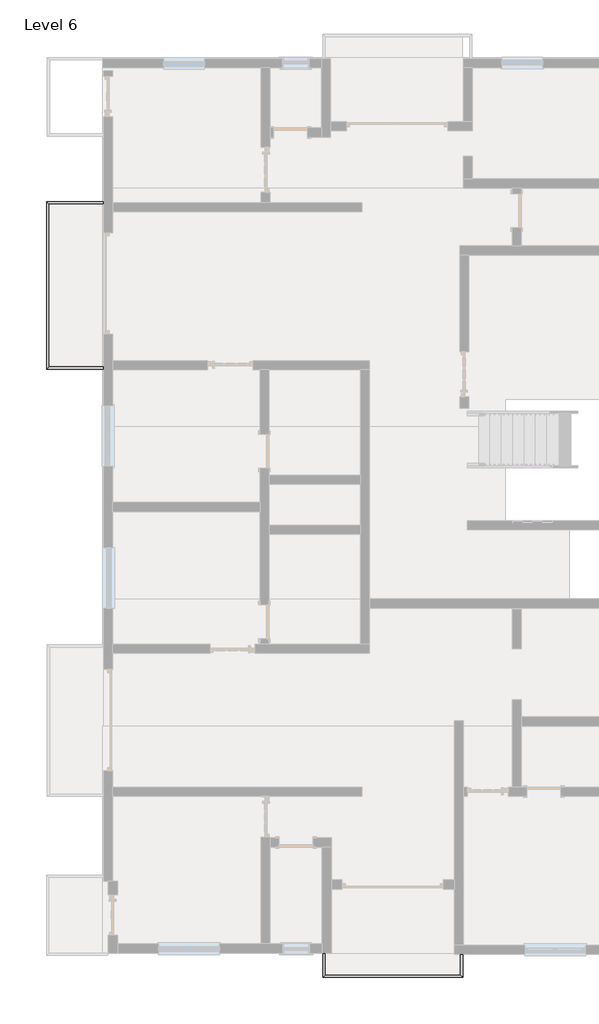
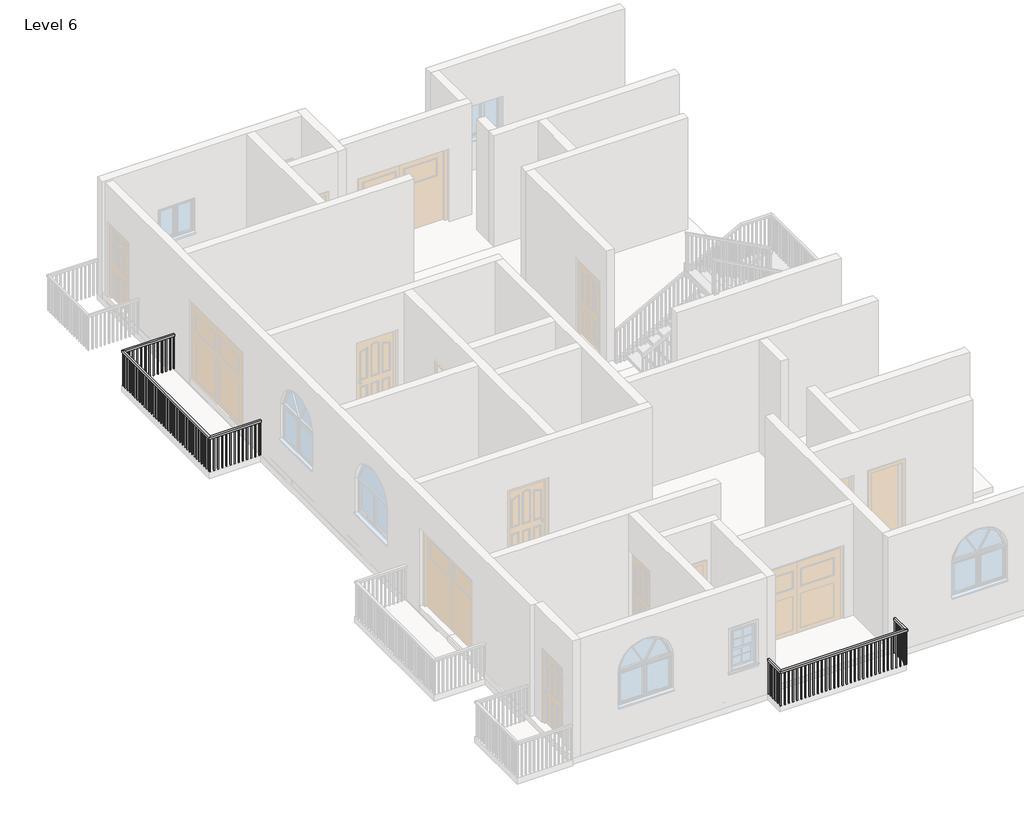
# One storey, part 4 of 7: 2 railings.
"""IFC4 building model written with IfcOpenShell, lengths in millimetres."""

from ifc_helpers import new_model, si_unit, frame, origin, place, context, project, spatial, polyline, outline, extrude, faceted_brep, element, save

model = new_model("IFC4")

# Units and contexts
model_context = context("Model", 3, world=origin())
ifc_project = project(units=[si_unit("LENGTHUNIT", "METRE", prefix="MILLI")], contexts=[model_context])

# Site, building, storey
site = spatial("IfcSite", under=ifc_project)
building = spatial("IfcBuilding", under=site)
storey = spatial("IfcBuildingStorey", under=building, Name="Level 6", Elevation=15240.0)

# Railings
placement = place(None, origin())
element("IfcRailing", 1, ObjectType="Handrail - Rectangular", at=placement, inside=storey, context=model_context, shape_type="SolidModel", body=[
    faceted_brep([(-1375.8109037, -10612.9037749, 16154.4), (-1375.8109037, -10612.9037749, 16103.6), (-1426.6109037, -10612.9037749, 16103.6), (-1426.6109037, -10612.9037749, 16154.4), (-1375.8109037, -11108.2037749, 16154.4), (-1375.8109037, -11108.2037749, 16103.6), (-1426.6109037, -11159.0037749, 16103.6), (-1426.6109037, -11159.0037749, 16154.4), (1659.4890963, -11108.2037749, 16154.4), (1659.4890963, -11108.2037749, 16103.6), (1710.2890963, -11159.0037749, 16103.6), (1710.2890963, -11159.0037749, 16154.4), (1659.4890963, -10638.3037749, 16154.4), (1710.2890963, -10638.3037749, 16154.4), (1710.2890963, -10638.3037749, 16103.6), (1659.4890963, -10638.3037749, 16103.6)], [[[0, 1, 2, 3]], [[1, 0, 4, 5]], [[2, 1, 5, 6]], [[3, 2, 6, 7]], [[0, 3, 7, 4]], [[5, 4, 8, 9]], [[6, 5, 9, 10]], [[7, 6, 10, 11]], [[4, 7, 11, 8]], [[12, 13, 14, 15]], [[9, 8, 12, 15]], [[10, 9, 15, 14]], [[11, 10, 14, 13]], [[8, 11, 13, 12]]]),
    extrude(outline(polyline([(1694.4140963, -10736.7287749), (1675.3640963, -10736.7287749), (1675.3640963, -10717.6787749), (1694.4140963, -10717.6787749), (1694.4140963, -10736.7287749)])), frame((0.0, 0.0, 15240.0), z_axis=(0.0, 0.0, 1.0), x_axis=(1.0, 0.0, 0.0)), (0.0, 0.0, 1.0), 863.6),
    extrude(outline(polyline([(1694.4140963, -10838.3287749), (1675.3640963, -10838.3287749), (1675.3640963, -10819.2787749), (1694.4140963, -10819.2787749), (1694.4140963, -10838.3287749)])), frame((0.0, 0.0, 15240.0), z_axis=(0.0, 0.0, 1.0), x_axis=(1.0, 0.0, 0.0)), (0.0, 0.0, 1.0), 863.6),
    extrude(outline(polyline([(1694.4140963, -10939.9287749), (1675.3640963, -10939.9287749), (1675.3640963, -10920.8787749), (1694.4140963, -10920.8787749), (1694.4140963, -10939.9287749)])), frame((0.0, 0.0, 15240.0), z_axis=(0.0, 0.0, 1.0), x_axis=(1.0, 0.0, 0.0)), (0.0, 0.0, 1.0), 863.6),
    extrude(outline(polyline([(1694.4140963, -11041.5287749), (1675.3640963, -11041.5287749), (1675.3640963, -11022.4787749), (1694.4140963, -11022.4787749), (1694.4140963, -11041.5287749)])), frame((0.0, 0.0, 15240.0), z_axis=(0.0, 0.0, 1.0), x_axis=(1.0, 0.0, 0.0)), (0.0, 0.0, 1.0), 863.6),
    extrude(outline(polyline([(1637.2640963, -11143.1287749), (1637.2640963, -11124.0787749), (1656.3140963, -11124.0787749), (1656.3140963, -11143.1287749), (1637.2640963, -11143.1287749)])), frame((0.0, 0.0, 15240.0), z_axis=(0.0, 0.0, 1.0), x_axis=(1.0, 0.0, 0.0)), (0.0, 0.0, 1.0), 863.6),
    extrude(outline(polyline([(1535.6640963, -11143.1287749), (1535.6640963, -11124.0787749), (1554.7140963, -11124.0787749), (1554.7140963, -11143.1287749), (1535.6640963, -11143.1287749)])), frame((0.0, 0.0, 15240.0), z_axis=(0.0, 0.0, 1.0), x_axis=(1.0, 0.0, 0.0)), (0.0, 0.0, 1.0), 863.6),
    extrude(outline(polyline([(1434.0640963, -11143.1287749), (1434.0640963, -11124.0787749), (1453.1140963, -11124.0787749), (1453.1140963, -11143.1287749), (1434.0640963, -11143.1287749)])), frame((0.0, 0.0, 15240.0), z_axis=(0.0, 0.0, 1.0), x_axis=(1.0, 0.0, 0.0)), (0.0, 0.0, 1.0), 863.6),
    extrude(outline(polyline([(1332.4640963, -11143.1287749), (1332.4640963, -11124.0787749), (1351.5140963, -11124.0787749), (1351.5140963, -11143.1287749), (1332.4640963, -11143.1287749)])), frame((0.0, 0.0, 15240.0), z_axis=(0.0, 0.0, 1.0), x_axis=(1.0, 0.0, 0.0)), (0.0, 0.0, 1.0), 863.6),
    extrude(outline(polyline([(1230.8640963, -11143.1287749), (1230.8640963, -11124.0787749), (1249.9140963, -11124.0787749), (1249.9140963, -11143.1287749), (1230.8640963, -11143.1287749)])), frame((0.0, 0.0, 15240.0), z_axis=(0.0, 0.0, 1.0), x_axis=(1.0, 0.0, 0.0)), (0.0, 0.0, 1.0), 863.6),
    extrude(outline(polyline([(1129.2640963, -11143.1287749), (1129.2640963, -11124.0787749), (1148.3140963, -11124.0787749), (1148.3140963, -11143.1287749), (1129.2640963, -11143.1287749)])), frame((0.0, 0.0, 15240.0), z_axis=(0.0, 0.0, 1.0), x_axis=(1.0, 0.0, 0.0)), (0.0, 0.0, 1.0), 863.6),
    extrude(outline(polyline([(1027.6640963, -11143.1287749), (1027.6640963, -11124.0787749), (1046.7140963, -11124.0787749), (1046.7140963, -11143.1287749), (1027.6640963, -11143.1287749)])), frame((0.0, 0.0, 15240.0), z_axis=(0.0, 0.0, 1.0), x_axis=(1.0, 0.0, 0.0)), (0.0, 0.0, 1.0), 863.6),
    extrude(outline(polyline([(926.0640963, -11143.1287749), (926.0640963, -11124.0787749), (945.1140963, -11124.0787749), (945.1140963, -11143.1287749), (926.0640963, -11143.1287749)])), frame((0.0, 0.0, 15240.0), z_axis=(0.0, 0.0, 1.0), x_axis=(1.0, 0.0, 0.0)), (0.0, 0.0, 1.0), 863.6),
    extrude(outline(polyline([(824.4640963, -11143.1287749), (824.4640963, -11124.0787749), (843.5140963, -11124.0787749), (843.5140963, -11143.1287749), (824.4640963, -11143.1287749)])), frame((0.0, 0.0, 15240.0), z_axis=(0.0, 0.0, 1.0), x_axis=(1.0, 0.0, 0.0)), (0.0, 0.0, 1.0), 863.6),
    extrude(outline(polyline([(722.8640963, -11143.1287749), (722.8640963, -11124.0787749), (741.9140963, -11124.0787749), (741.9140963, -11143.1287749), (722.8640963, -11143.1287749)])), frame((0.0, 0.0, 15240.0), z_axis=(0.0, 0.0, 1.0), x_axis=(1.0, 0.0, 0.0)), (0.0, 0.0, 1.0), 863.6),
    extrude(outline(polyline([(621.2640963, -11143.1287749), (621.2640963, -11124.0787749), (640.3140963, -11124.0787749), (640.3140963, -11143.1287749), (621.2640963, -11143.1287749)])), frame((0.0, 0.0, 15240.0), z_axis=(0.0, 0.0, 1.0), x_axis=(1.0, 0.0, 0.0)), (0.0, 0.0, 1.0), 863.6),
    extrude(outline(polyline([(519.6640963, -11143.1287749), (519.6640963, -11124.0787749), (538.7140963, -11124.0787749), (538.7140963, -11143.1287749), (519.6640963, -11143.1287749)])), frame((0.0, 0.0, 15240.0), z_axis=(0.0, 0.0, 1.0), x_axis=(1.0, 0.0, 0.0)), (0.0, 0.0, 1.0), 863.6),
    extrude(outline(polyline([(418.0640963, -11143.1287749), (418.0640963, -11124.0787749), (437.1140963, -11124.0787749), (437.1140963, -11143.1287749), (418.0640963, -11143.1287749)])), frame((0.0, 0.0, 15240.0), z_axis=(0.0, 0.0, 1.0), x_axis=(1.0, 0.0, 0.0)), (0.0, 0.0, 1.0), 863.6),
    extrude(outline(polyline([(316.4640963, -11143.1287749), (316.4640963, -11124.0787749), (335.5140963, -11124.0787749), (335.5140963, -11143.1287749), (316.4640963, -11143.1287749)])), frame((0.0, 0.0, 15240.0), z_axis=(0.0, 0.0, 1.0), x_axis=(1.0, 0.0, 0.0)), (0.0, 0.0, 1.0), 863.6),
    extrude(outline(polyline([(214.8640963, -11143.1287749), (214.8640963, -11124.0787749), (233.9140963, -11124.0787749), (233.9140963, -11143.1287749), (214.8640963, -11143.1287749)])), frame((0.0, 0.0, 15240.0), z_axis=(0.0, 0.0, 1.0), x_axis=(1.0, 0.0, 0.0)), (0.0, 0.0, 1.0), 863.6),
    extrude(outline(polyline([(113.2640963, -11143.1287749), (113.2640963, -11124.0787749), (132.3140963, -11124.0787749), (132.3140963, -11143.1287749), (113.2640963, -11143.1287749)])), frame((0.0, 0.0, 15240.0), z_axis=(0.0, 0.0, 1.0), x_axis=(1.0, 0.0, 0.0)), (0.0, 0.0, 1.0), 863.6),
    extrude(outline(polyline([(11.6640963, -11143.1287749), (11.6640963, -11124.0787749), (30.7140963, -11124.0787749), (30.7140963, -11143.1287749), (11.6640963, -11143.1287749)])), frame((0.0, 0.0, 15240.0), z_axis=(0.0, 0.0, 1.0), x_axis=(1.0, 0.0, 0.0)), (0.0, 0.0, 1.0), 863.6),
    extrude(outline(polyline([(-89.9359037, -11143.1287749), (-89.9359037, -11124.0787749), (-70.8859037, -11124.0787749), (-70.8859037, -11143.1287749), (-89.9359037, -11143.1287749)])), frame((0.0, 0.0, 15240.0), z_axis=(0.0, 0.0, 1.0), x_axis=(1.0, 0.0, 0.0)), (0.0, 0.0, 1.0), 863.6),
    extrude(outline(polyline([(-191.5359037, -11143.1287749), (-191.5359037, -11124.0787749), (-172.4859037, -11124.0787749), (-172.4859037, -11143.1287749), (-191.5359037, -11143.1287749)])), frame((0.0, 0.0, 15240.0), z_axis=(0.0, 0.0, 1.0), x_axis=(1.0, 0.0, 0.0)), (0.0, 0.0, 1.0), 863.6),
    extrude(outline(polyline([(-293.1359037, -11143.1287749), (-293.1359037, -11124.0787749), (-274.0859037, -11124.0787749), (-274.0859037, -11143.1287749), (-293.1359037, -11143.1287749)])), frame((0.0, 0.0, 15240.0), z_axis=(0.0, 0.0, 1.0), x_axis=(1.0, 0.0, 0.0)), (0.0, 0.0, 1.0), 863.6),
    extrude(outline(polyline([(-394.7359037, -11143.1287749), (-394.7359037, -11124.0787749), (-375.6859037, -11124.0787749), (-375.6859037, -11143.1287749), (-394.7359037, -11143.1287749)])), frame((0.0, 0.0, 15240.0), z_axis=(0.0, 0.0, 1.0), x_axis=(1.0, 0.0, 0.0)), (0.0, 0.0, 1.0), 863.6),
    extrude(outline(polyline([(-496.3359037, -11143.1287749), (-496.3359037, -11124.0787749), (-477.2859037, -11124.0787749), (-477.2859037, -11143.1287749), (-496.3359037, -11143.1287749)])), frame((0.0, 0.0, 15240.0), z_axis=(0.0, 0.0, 1.0), x_axis=(1.0, 0.0, 0.0)), (0.0, 0.0, 1.0), 863.6),
    extrude(outline(polyline([(-597.9359037, -11143.1287749), (-597.9359037, -11124.0787749), (-578.8859037, -11124.0787749), (-578.8859037, -11143.1287749), (-597.9359037, -11143.1287749)])), frame((0.0, 0.0, 15240.0), z_axis=(0.0, 0.0, 1.0), x_axis=(1.0, 0.0, 0.0)), (0.0, 0.0, 1.0), 863.6),
    extrude(outline(polyline([(-699.5359037, -11143.1287749), (-699.5359037, -11124.0787749), (-680.4859037, -11124.0787749), (-680.4859037, -11143.1287749), (-699.5359037, -11143.1287749)])), frame((0.0, 0.0, 15240.0), z_axis=(0.0, 0.0, 1.0), x_axis=(1.0, 0.0, 0.0)), (0.0, 0.0, 1.0), 863.6),
    extrude(outline(polyline([(-801.1359037, -11143.1287749), (-801.1359037, -11124.0787749), (-782.0859037, -11124.0787749), (-782.0859037, -11143.1287749), (-801.1359037, -11143.1287749)])), frame((0.0, 0.0, 15240.0), z_axis=(0.0, 0.0, 1.0), x_axis=(1.0, 0.0, 0.0)), (0.0, 0.0, 1.0), 863.6),
    extrude(outline(polyline([(-902.7359037, -11143.1287749), (-902.7359037, -11124.0787749), (-883.6859037, -11124.0787749), (-883.6859037, -11143.1287749), (-902.7359037, -11143.1287749)])), frame((0.0, 0.0, 15240.0), z_axis=(0.0, 0.0, 1.0), x_axis=(1.0, 0.0, 0.0)), (0.0, 0.0, 1.0), 863.6),
    extrude(outline(polyline([(-1004.3359037, -11143.1287749), (-1004.3359037, -11124.0787749), (-985.2859037, -11124.0787749), (-985.2859037, -11143.1287749), (-1004.3359037, -11143.1287749)])), frame((0.0, 0.0, 15240.0), z_axis=(0.0, 0.0, 1.0), x_axis=(1.0, 0.0, 0.0)), (0.0, 0.0, 1.0), 863.6),
    extrude(outline(polyline([(-1105.9359037, -11143.1287749), (-1105.9359037, -11124.0787749), (-1086.8859037, -11124.0787749), (-1086.8859037, -11143.1287749), (-1105.9359037, -11143.1287749)])), frame((0.0, 0.0, 15240.0), z_axis=(0.0, 0.0, 1.0), x_axis=(1.0, 0.0, 0.0)), (0.0, 0.0, 1.0), 863.6),
    extrude(outline(polyline([(-1207.5359037, -11143.1287749), (-1207.5359037, -11124.0787749), (-1188.4859037, -11124.0787749), (-1188.4859037, -11143.1287749), (-1207.5359037, -11143.1287749)])), frame((0.0, 0.0, 15240.0), z_axis=(0.0, 0.0, 1.0), x_axis=(1.0, 0.0, 0.0)), (0.0, 0.0, 1.0), 863.6),
    extrude(outline(polyline([(-1309.1359037, -11143.1287749), (-1309.1359037, -11124.0787749), (-1290.0859037, -11124.0787749), (-1290.0859037, -11143.1287749), (-1309.1359037, -11143.1287749)])), frame((0.0, 0.0, 15240.0), z_axis=(0.0, 0.0, 1.0), x_axis=(1.0, 0.0, 0.0)), (0.0, 0.0, 1.0), 863.6),
    extrude(outline(polyline([(-1410.7359037, -11111.3787749), (-1391.6859037, -11111.3787749), (-1391.6859037, -11130.4287749), (-1410.7359037, -11130.4287749), (-1410.7359037, -11111.3787749)])), frame((0.0, 0.0, 15240.0), z_axis=(0.0, 0.0, 1.0), x_axis=(1.0, 0.0, 0.0)), (0.0, 0.0, 1.0), 863.6),
    extrude(outline(polyline([(-1410.7359037, -11009.7787749), (-1391.6859037, -11009.7787749), (-1391.6859037, -11028.8287749), (-1410.7359037, -11028.8287749), (-1410.7359037, -11009.7787749)])), frame((0.0, 0.0, 15240.0), z_axis=(0.0, 0.0, 1.0), x_axis=(1.0, 0.0, 0.0)), (0.0, 0.0, 1.0), 863.6),
    extrude(outline(polyline([(-1410.7359037, -10908.1787749), (-1391.6859037, -10908.1787749), (-1391.6859037, -10927.2287749), (-1410.7359037, -10927.2287749), (-1410.7359037, -10908.1787749)])), frame((0.0, 0.0, 15240.0), z_axis=(0.0, 0.0, 1.0), x_axis=(1.0, 0.0, 0.0)), (0.0, 0.0, 1.0), 863.6),
    extrude(outline(polyline([(-1410.7359037, -10806.5787749), (-1391.6859037, -10806.5787749), (-1391.6859037, -10825.6287749), (-1410.7359037, -10825.6287749), (-1410.7359037, -10806.5787749)])), frame((0.0, 0.0, 15240.0), z_axis=(0.0, 0.0, 1.0), x_axis=(1.0, 0.0, 0.0)), (0.0, 0.0, 1.0), 863.6),
    extrude(outline(polyline([(-1410.7359037, -10704.9787749), (-1391.6859037, -10704.9787749), (-1391.6859037, -10724.0287749), (-1410.7359037, -10724.0287749), (-1410.7359037, -10704.9787749)])), frame((0.0, 0.0, 15240.0), z_axis=(0.0, 0.0, 1.0), x_axis=(1.0, 0.0, 0.0)), (0.0, 0.0, 1.0), 863.6),
    extrude(outline(polyline([(1675.3640963, -11143.1287749), (1675.3640963, -11124.0787749), (1694.4140963, -11124.0787749), (1694.4140963, -11143.1287749), (1675.3640963, -11143.1287749)])), frame((0.0, 0.0, 15240.0), z_axis=(0.0, 0.0, 1.0), x_axis=(1.0, 0.0, 0.0)), (0.0, 0.0, 1.0), 863.6),
    extrude(outline(polyline([(-1410.7359037, -11124.0787749), (-1391.6859037, -11124.0787749), (-1391.6859037, -11143.1287749), (-1410.7359037, -11143.1287749), (-1410.7359037, -11124.0787749)])), frame((0.0, 0.0, 15240.0), z_axis=(0.0, 0.0, 1.0), x_axis=(1.0, 0.0, 0.0)), (0.0, 0.0, 1.0), 863.6),
    extrude(outline(polyline([(1694.4140963, -10657.3537749), (1675.3640963, -10657.3537749), (1675.3640963, -10638.3037749), (1694.4140963, -10638.3037749), (1694.4140963, -10657.3537749)])), frame((0.0, 0.0, 15240.0), z_axis=(0.0, 0.0, 1.0), x_axis=(1.0, 0.0, 0.0)), (0.0, 0.0, 1.0), 863.6),
    extrude(outline(polyline([(-1410.7359037, -10612.9037749), (-1391.6859037, -10612.9037749), (-1391.6859037, -10631.9537749), (-1410.7359037, -10631.9537749), (-1410.7359037, -10612.9037749)])), frame((0.0, 0.0, 15240.0), z_axis=(0.0, 0.0, 1.0), x_axis=(1.0, 0.0, 0.0)), (0.0, 0.0, 1.0), 863.6),
])
element("IfcRailing", 2, ObjectType="Handrail - Rectangular", at=placement, inside=storey, context=model_context, shape_type="SolidModel", body=[
    faceted_brep([(-6330.8013636, 6151.0962251, 16154.4), (-6330.8013636, 6151.0962251, 16103.6), (-6330.8013636, 6201.8962251, 16103.6), (-6330.8013636, 6201.8962251, 16154.4), (-7563.8859037, 6151.0962251, 16154.4), (-7563.8859037, 6151.0962251, 16103.6), (-7614.6859037, 6201.8962251, 16103.6), (-7614.6859037, 6201.8962251, 16154.4), (-7563.8859037, 2506.1962251, 16154.4), (-7563.8859037, 2506.1962251, 16103.6), (-7614.6859037, 2455.3962251, 16103.6), (-7614.6859037, 2455.3962251, 16154.4), (-6330.8013636, 2506.1962251, 16154.4), (-6330.8013636, 2455.3962251, 16154.4), (-6330.8013636, 2455.3962251, 16103.6), (-6330.8013636, 2506.1962251, 16103.6)], [[[0, 1, 2, 3]], [[1, 0, 4, 5]], [[2, 1, 5, 6]], [[3, 2, 6, 7]], [[0, 3, 7, 4]], [[5, 4, 8, 9]], [[6, 5, 9, 10]], [[7, 6, 10, 11]], [[4, 7, 11, 8]], [[12, 13, 14, 15]], [[9, 8, 12, 15]], [[10, 9, 15, 14]], [[11, 10, 14, 13]], [[8, 11, 13, 12]]]),
    extrude(outline(polyline([(-6379.6109037, 2471.2712251), (-6379.6109037, 2490.3212251), (-6360.5609037, 2490.3212251), (-6360.5609037, 2471.2712251), (-6379.6109037, 2471.2712251)])), frame((0.0, 0.0, 15240.0), z_axis=(0.0, 0.0, 1.0), x_axis=(1.0, 0.0, 0.0)), (0.0, 0.0, 1.0), 863.6),
    extrude(outline(polyline([(-6481.2109037, 2471.2712251), (-6481.2109037, 2490.3212251), (-6462.1609037, 2490.3212251), (-6462.1609037, 2471.2712251), (-6481.2109037, 2471.2712251)])), frame((0.0, 0.0, 15240.0), z_axis=(0.0, 0.0, 1.0), x_axis=(1.0, 0.0, 0.0)), (0.0, 0.0, 1.0), 863.6),
    extrude(outline(polyline([(-6582.8109037, 2471.2712251), (-6582.8109037, 2490.3212251), (-6563.7609037, 2490.3212251), (-6563.7609037, 2471.2712251), (-6582.8109037, 2471.2712251)])), frame((0.0, 0.0, 15240.0), z_axis=(0.0, 0.0, 1.0), x_axis=(1.0, 0.0, 0.0)), (0.0, 0.0, 1.0), 863.6),
    extrude(outline(polyline([(-6684.4109037, 2471.2712251), (-6684.4109037, 2490.3212251), (-6665.3609037, 2490.3212251), (-6665.3609037, 2471.2712251), (-6684.4109037, 2471.2712251)])), frame((0.0, 0.0, 15240.0), z_axis=(0.0, 0.0, 1.0), x_axis=(1.0, 0.0, 0.0)), (0.0, 0.0, 1.0), 863.6),
    extrude(outline(polyline([(-6786.0109037, 2471.2712251), (-6786.0109037, 2490.3212251), (-6766.9609037, 2490.3212251), (-6766.9609037, 2471.2712251), (-6786.0109037, 2471.2712251)])), frame((0.0, 0.0, 15240.0), z_axis=(0.0, 0.0, 1.0), x_axis=(1.0, 0.0, 0.0)), (0.0, 0.0, 1.0), 863.6),
    extrude(outline(polyline([(-6887.6109037, 2471.2712251), (-6887.6109037, 2490.3212251), (-6868.5609037, 2490.3212251), (-6868.5609037, 2471.2712251), (-6887.6109037, 2471.2712251)])), frame((0.0, 0.0, 15240.0), z_axis=(0.0, 0.0, 1.0), x_axis=(1.0, 0.0, 0.0)), (0.0, 0.0, 1.0), 863.6),
    extrude(outline(polyline([(-6989.2109037, 2471.2712251), (-6989.2109037, 2490.3212251), (-6970.1609037, 2490.3212251), (-6970.1609037, 2471.2712251), (-6989.2109037, 2471.2712251)])), frame((0.0, 0.0, 15240.0), z_axis=(0.0, 0.0, 1.0), x_axis=(1.0, 0.0, 0.0)), (0.0, 0.0, 1.0), 863.6),
    extrude(outline(polyline([(-7090.8109037, 2471.2712251), (-7090.8109037, 2490.3212251), (-7071.7609037, 2490.3212251), (-7071.7609037, 2471.2712251), (-7090.8109037, 2471.2712251)])), frame((0.0, 0.0, 15240.0), z_axis=(0.0, 0.0, 1.0), x_axis=(1.0, 0.0, 0.0)), (0.0, 0.0, 1.0), 863.6),
    extrude(outline(polyline([(-7192.4109037, 2471.2712251), (-7192.4109037, 2490.3212251), (-7173.3609037, 2490.3212251), (-7173.3609037, 2471.2712251), (-7192.4109037, 2471.2712251)])), frame((0.0, 0.0, 15240.0), z_axis=(0.0, 0.0, 1.0), x_axis=(1.0, 0.0, 0.0)), (0.0, 0.0, 1.0), 863.6),
    extrude(outline(polyline([(-7294.0109037, 2471.2712251), (-7294.0109037, 2490.3212251), (-7274.9609037, 2490.3212251), (-7274.9609037, 2471.2712251), (-7294.0109037, 2471.2712251)])), frame((0.0, 0.0, 15240.0), z_axis=(0.0, 0.0, 1.0), x_axis=(1.0, 0.0, 0.0)), (0.0, 0.0, 1.0), 863.6),
    extrude(outline(polyline([(-7395.6109037, 2471.2712251), (-7395.6109037, 2490.3212251), (-7376.5609037, 2490.3212251), (-7376.5609037, 2471.2712251), (-7395.6109037, 2471.2712251)])), frame((0.0, 0.0, 15240.0), z_axis=(0.0, 0.0, 1.0), x_axis=(1.0, 0.0, 0.0)), (0.0, 0.0, 1.0), 863.6),
    extrude(outline(polyline([(-7497.2109037, 2471.2712251), (-7497.2109037, 2490.3212251), (-7478.1609037, 2490.3212251), (-7478.1609037, 2471.2712251), (-7497.2109037, 2471.2712251)])), frame((0.0, 0.0, 15240.0), z_axis=(0.0, 0.0, 1.0), x_axis=(1.0, 0.0, 0.0)), (0.0, 0.0, 1.0), 863.6),
    extrude(outline(polyline([(-7598.8109037, 2528.4212251), (-7579.7609037, 2528.4212251), (-7579.7609037, 2509.3712251), (-7598.8109037, 2509.3712251), (-7598.8109037, 2528.4212251)])), frame((0.0, 0.0, 15240.0), z_axis=(0.0, 0.0, 1.0), x_axis=(1.0, 0.0, 0.0)), (0.0, 0.0, 1.0), 863.6),
    extrude(outline(polyline([(-7598.8109037, 2630.0212251), (-7579.7609037, 2630.0212251), (-7579.7609037, 2610.9712251), (-7598.8109037, 2610.9712251), (-7598.8109037, 2630.0212251)])), frame((0.0, 0.0, 15240.0), z_axis=(0.0, 0.0, 1.0), x_axis=(1.0, 0.0, 0.0)), (0.0, 0.0, 1.0), 863.6),
    extrude(outline(polyline([(-7598.8109037, 2731.6212251), (-7579.7609037, 2731.6212251), (-7579.7609037, 2712.5712251), (-7598.8109037, 2712.5712251), (-7598.8109037, 2731.6212251)])), frame((0.0, 0.0, 15240.0), z_axis=(0.0, 0.0, 1.0), x_axis=(1.0, 0.0, 0.0)), (0.0, 0.0, 1.0), 863.6),
    extrude(outline(polyline([(-7598.8109037, 2833.2212251), (-7579.7609037, 2833.2212251), (-7579.7609037, 2814.1712251), (-7598.8109037, 2814.1712251), (-7598.8109037, 2833.2212251)])), frame((0.0, 0.0, 15240.0), z_axis=(0.0, 0.0, 1.0), x_axis=(1.0, 0.0, 0.0)), (0.0, 0.0, 1.0), 863.6),
    extrude(outline(polyline([(-7598.8109037, 2934.8212251), (-7579.7609037, 2934.8212251), (-7579.7609037, 2915.7712251), (-7598.8109037, 2915.7712251), (-7598.8109037, 2934.8212251)])), frame((0.0, 0.0, 15240.0), z_axis=(0.0, 0.0, 1.0), x_axis=(1.0, 0.0, 0.0)), (0.0, 0.0, 1.0), 863.6),
    extrude(outline(polyline([(-7598.8109037, 3036.4212251), (-7579.7609037, 3036.4212251), (-7579.7609037, 3017.3712251), (-7598.8109037, 3017.3712251), (-7598.8109037, 3036.4212251)])), frame((0.0, 0.0, 15240.0), z_axis=(0.0, 0.0, 1.0), x_axis=(1.0, 0.0, 0.0)), (0.0, 0.0, 1.0), 863.6),
    extrude(outline(polyline([(-7598.8109037, 3138.0212251), (-7579.7609037, 3138.0212251), (-7579.7609037, 3118.9712251), (-7598.8109037, 3118.9712251), (-7598.8109037, 3138.0212251)])), frame((0.0, 0.0, 15240.0), z_axis=(0.0, 0.0, 1.0), x_axis=(1.0, 0.0, 0.0)), (0.0, 0.0, 1.0), 863.6),
    extrude(outline(polyline([(-7598.8109037, 3239.6212251), (-7579.7609037, 3239.6212251), (-7579.7609037, 3220.5712251), (-7598.8109037, 3220.5712251), (-7598.8109037, 3239.6212251)])), frame((0.0, 0.0, 15240.0), z_axis=(0.0, 0.0, 1.0), x_axis=(1.0, 0.0, 0.0)), (0.0, 0.0, 1.0), 863.6),
    extrude(outline(polyline([(-7598.8109037, 3341.2212251), (-7579.7609037, 3341.2212251), (-7579.7609037, 3322.1712251), (-7598.8109037, 3322.1712251), (-7598.8109037, 3341.2212251)])), frame((0.0, 0.0, 15240.0), z_axis=(0.0, 0.0, 1.0), x_axis=(1.0, 0.0, 0.0)), (0.0, 0.0, 1.0), 863.6),
    extrude(outline(polyline([(-7598.8109037, 3442.8212251), (-7579.7609037, 3442.8212251), (-7579.7609037, 3423.7712251), (-7598.8109037, 3423.7712251), (-7598.8109037, 3442.8212251)])), frame((0.0, 0.0, 15240.0), z_axis=(0.0, 0.0, 1.0), x_axis=(1.0, 0.0, 0.0)), (0.0, 0.0, 1.0), 863.6),
    extrude(outline(polyline([(-7598.8109037, 3544.4212251), (-7579.7609037, 3544.4212251), (-7579.7609037, 3525.3712251), (-7598.8109037, 3525.3712251), (-7598.8109037, 3544.4212251)])), frame((0.0, 0.0, 15240.0), z_axis=(0.0, 0.0, 1.0), x_axis=(1.0, 0.0, 0.0)), (0.0, 0.0, 1.0), 863.6),
    extrude(outline(polyline([(-7598.8109037, 3646.0212251), (-7579.7609037, 3646.0212251), (-7579.7609037, 3626.9712251), (-7598.8109037, 3626.9712251), (-7598.8109037, 3646.0212251)])), frame((0.0, 0.0, 15240.0), z_axis=(0.0, 0.0, 1.0), x_axis=(1.0, 0.0, 0.0)), (0.0, 0.0, 1.0), 863.6),
    extrude(outline(polyline([(-7598.8109037, 3747.6212251), (-7579.7609037, 3747.6212251), (-7579.7609037, 3728.5712251), (-7598.8109037, 3728.5712251), (-7598.8109037, 3747.6212251)])), frame((0.0, 0.0, 15240.0), z_axis=(0.0, 0.0, 1.0), x_axis=(1.0, 0.0, 0.0)), (0.0, 0.0, 1.0), 863.6),
    extrude(outline(polyline([(-7598.8109037, 3849.2212251), (-7579.7609037, 3849.2212251), (-7579.7609037, 3830.1712251), (-7598.8109037, 3830.1712251), (-7598.8109037, 3849.2212251)])), frame((0.0, 0.0, 15240.0), z_axis=(0.0, 0.0, 1.0), x_axis=(1.0, 0.0, 0.0)), (0.0, 0.0, 1.0), 863.6),
    extrude(outline(polyline([(-7598.8109037, 3950.8212251), (-7579.7609037, 3950.8212251), (-7579.7609037, 3931.7712251), (-7598.8109037, 3931.7712251), (-7598.8109037, 3950.8212251)])), frame((0.0, 0.0, 15240.0), z_axis=(0.0, 0.0, 1.0), x_axis=(1.0, 0.0, 0.0)), (0.0, 0.0, 1.0), 863.6),
    extrude(outline(polyline([(-7598.8109037, 4052.4212251), (-7579.7609037, 4052.4212251), (-7579.7609037, 4033.3712251), (-7598.8109037, 4033.3712251), (-7598.8109037, 4052.4212251)])), frame((0.0, 0.0, 15240.0), z_axis=(0.0, 0.0, 1.0), x_axis=(1.0, 0.0, 0.0)), (0.0, 0.0, 1.0), 863.6),
    extrude(outline(polyline([(-7598.8109037, 4154.0212251), (-7579.7609037, 4154.0212251), (-7579.7609037, 4134.9712251), (-7598.8109037, 4134.9712251), (-7598.8109037, 4154.0212251)])), frame((0.0, 0.0, 15240.0), z_axis=(0.0, 0.0, 1.0), x_axis=(1.0, 0.0, 0.0)), (0.0, 0.0, 1.0), 863.6),
    extrude(outline(polyline([(-7598.8109037, 4255.6212251), (-7579.7609037, 4255.6212251), (-7579.7609037, 4236.5712251), (-7598.8109037, 4236.5712251), (-7598.8109037, 4255.6212251)])), frame((0.0, 0.0, 15240.0), z_axis=(0.0, 0.0, 1.0), x_axis=(1.0, 0.0, 0.0)), (0.0, 0.0, 1.0), 863.6),
    extrude(outline(polyline([(-7598.8109037, 4357.2212251), (-7579.7609037, 4357.2212251), (-7579.7609037, 4338.1712251), (-7598.8109037, 4338.1712251), (-7598.8109037, 4357.2212251)])), frame((0.0, 0.0, 15240.0), z_axis=(0.0, 0.0, 1.0), x_axis=(1.0, 0.0, 0.0)), (0.0, 0.0, 1.0), 863.6),
    extrude(outline(polyline([(-7598.8109037, 4458.8212251), (-7579.7609037, 4458.8212251), (-7579.7609037, 4439.7712251), (-7598.8109037, 4439.7712251), (-7598.8109037, 4458.8212251)])), frame((0.0, 0.0, 15240.0), z_axis=(0.0, 0.0, 1.0), x_axis=(1.0, 0.0, 0.0)), (0.0, 0.0, 1.0), 863.6),
    extrude(outline(polyline([(-7598.8109037, 4560.4212251), (-7579.7609037, 4560.4212251), (-7579.7609037, 4541.3712251), (-7598.8109037, 4541.3712251), (-7598.8109037, 4560.4212251)])), frame((0.0, 0.0, 15240.0), z_axis=(0.0, 0.0, 1.0), x_axis=(1.0, 0.0, 0.0)), (0.0, 0.0, 1.0), 863.6),
    extrude(outline(polyline([(-7598.8109037, 4662.0212251), (-7579.7609037, 4662.0212251), (-7579.7609037, 4642.9712251), (-7598.8109037, 4642.9712251), (-7598.8109037, 4662.0212251)])), frame((0.0, 0.0, 15240.0), z_axis=(0.0, 0.0, 1.0), x_axis=(1.0, 0.0, 0.0)), (0.0, 0.0, 1.0), 863.6),
    extrude(outline(polyline([(-7598.8109037, 4763.6212251), (-7579.7609037, 4763.6212251), (-7579.7609037, 4744.5712251), (-7598.8109037, 4744.5712251), (-7598.8109037, 4763.6212251)])), frame((0.0, 0.0, 15240.0), z_axis=(0.0, 0.0, 1.0), x_axis=(1.0, 0.0, 0.0)), (0.0, 0.0, 1.0), 863.6),
    extrude(outline(polyline([(-7598.8109037, 4865.2212251), (-7579.7609037, 4865.2212251), (-7579.7609037, 4846.1712251), (-7598.8109037, 4846.1712251), (-7598.8109037, 4865.2212251)])), frame((0.0, 0.0, 15240.0), z_axis=(0.0, 0.0, 1.0), x_axis=(1.0, 0.0, 0.0)), (0.0, 0.0, 1.0), 863.6),
    extrude(outline(polyline([(-7598.8109037, 4966.8212251), (-7579.7609037, 4966.8212251), (-7579.7609037, 4947.7712251), (-7598.8109037, 4947.7712251), (-7598.8109037, 4966.8212251)])), frame((0.0, 0.0, 15240.0), z_axis=(0.0, 0.0, 1.0), x_axis=(1.0, 0.0, 0.0)), (0.0, 0.0, 1.0), 863.6),
    extrude(outline(polyline([(-7598.8109037, 5068.4212251), (-7579.7609037, 5068.4212251), (-7579.7609037, 5049.3712251), (-7598.8109037, 5049.3712251), (-7598.8109037, 5068.4212251)])), frame((0.0, 0.0, 15240.0), z_axis=(0.0, 0.0, 1.0), x_axis=(1.0, 0.0, 0.0)), (0.0, 0.0, 1.0), 863.6),
    extrude(outline(polyline([(-7598.8109037, 5170.0212251), (-7579.7609037, 5170.0212251), (-7579.7609037, 5150.9712251), (-7598.8109037, 5150.9712251), (-7598.8109037, 5170.0212251)])), frame((0.0, 0.0, 15240.0), z_axis=(0.0, 0.0, 1.0), x_axis=(1.0, 0.0, 0.0)), (0.0, 0.0, 1.0), 863.6),
    extrude(outline(polyline([(-7598.8109037, 5271.6212251), (-7579.7609037, 5271.6212251), (-7579.7609037, 5252.5712251), (-7598.8109037, 5252.5712251), (-7598.8109037, 5271.6212251)])), frame((0.0, 0.0, 15240.0), z_axis=(0.0, 0.0, 1.0), x_axis=(1.0, 0.0, 0.0)), (0.0, 0.0, 1.0), 863.6),
    extrude(outline(polyline([(-7598.8109037, 5373.2212251), (-7579.7609037, 5373.2212251), (-7579.7609037, 5354.1712251), (-7598.8109037, 5354.1712251), (-7598.8109037, 5373.2212251)])), frame((0.0, 0.0, 15240.0), z_axis=(0.0, 0.0, 1.0), x_axis=(1.0, 0.0, 0.0)), (0.0, 0.0, 1.0), 863.6),
    extrude(outline(polyline([(-7598.8109037, 5474.8212251), (-7579.7609037, 5474.8212251), (-7579.7609037, 5455.7712251), (-7598.8109037, 5455.7712251), (-7598.8109037, 5474.8212251)])), frame((0.0, 0.0, 15240.0), z_axis=(0.0, 0.0, 1.0), x_axis=(1.0, 0.0, 0.0)), (0.0, 0.0, 1.0), 863.6),
    extrude(outline(polyline([(-7598.8109037, 5576.4212251), (-7579.7609037, 5576.4212251), (-7579.7609037, 5557.3712251), (-7598.8109037, 5557.3712251), (-7598.8109037, 5576.4212251)])), frame((0.0, 0.0, 15240.0), z_axis=(0.0, 0.0, 1.0), x_axis=(1.0, 0.0, 0.0)), (0.0, 0.0, 1.0), 863.6),
    extrude(outline(polyline([(-7598.8109037, 5678.0212251), (-7579.7609037, 5678.0212251), (-7579.7609037, 5658.9712251), (-7598.8109037, 5658.9712251), (-7598.8109037, 5678.0212251)])), frame((0.0, 0.0, 15240.0), z_axis=(0.0, 0.0, 1.0), x_axis=(1.0, 0.0, 0.0)), (0.0, 0.0, 1.0), 863.6),
    extrude(outline(polyline([(-7598.8109037, 5779.6212251), (-7579.7609037, 5779.6212251), (-7579.7609037, 5760.5712251), (-7598.8109037, 5760.5712251), (-7598.8109037, 5779.6212251)])), frame((0.0, 0.0, 15240.0), z_axis=(0.0, 0.0, 1.0), x_axis=(1.0, 0.0, 0.0)), (0.0, 0.0, 1.0), 863.6),
    extrude(outline(polyline([(-7598.8109037, 5881.2212251), (-7579.7609037, 5881.2212251), (-7579.7609037, 5862.1712251), (-7598.8109037, 5862.1712251), (-7598.8109037, 5881.2212251)])), frame((0.0, 0.0, 15240.0), z_axis=(0.0, 0.0, 1.0), x_axis=(1.0, 0.0, 0.0)), (0.0, 0.0, 1.0), 863.6),
    extrude(outline(polyline([(-7598.8109037, 5982.8212251), (-7579.7609037, 5982.8212251), (-7579.7609037, 5963.7712251), (-7598.8109037, 5963.7712251), (-7598.8109037, 5982.8212251)])), frame((0.0, 0.0, 15240.0), z_axis=(0.0, 0.0, 1.0), x_axis=(1.0, 0.0, 0.0)), (0.0, 0.0, 1.0), 863.6),
    extrude(outline(polyline([(-7598.8109037, 6084.4212251), (-7579.7609037, 6084.4212251), (-7579.7609037, 6065.3712251), (-7598.8109037, 6065.3712251), (-7598.8109037, 6084.4212251)])), frame((0.0, 0.0, 15240.0), z_axis=(0.0, 0.0, 1.0), x_axis=(1.0, 0.0, 0.0)), (0.0, 0.0, 1.0), 863.6),
    extrude(outline(polyline([(-7540.4763636, 6186.0212251), (-7540.4763636, 6166.9712251), (-7559.5263636, 6166.9712251), (-7559.5263636, 6186.0212251), (-7540.4763636, 6186.0212251)])), frame((0.0, 0.0, 15240.0), z_axis=(0.0, 0.0, 1.0), x_axis=(1.0, 0.0, 0.0)), (0.0, 0.0, 1.0), 863.6),
    extrude(outline(polyline([(-7438.8763636, 6186.0212251), (-7438.8763636, 6166.9712251), (-7457.9263636, 6166.9712251), (-7457.9263636, 6186.0212251), (-7438.8763636, 6186.0212251)])), frame((0.0, 0.0, 15240.0), z_axis=(0.0, 0.0, 1.0), x_axis=(1.0, 0.0, 0.0)), (0.0, 0.0, 1.0), 863.6),
    extrude(outline(polyline([(-7337.2763636, 6186.0212251), (-7337.2763636, 6166.9712251), (-7356.3263636, 6166.9712251), (-7356.3263636, 6186.0212251), (-7337.2763636, 6186.0212251)])), frame((0.0, 0.0, 15240.0), z_axis=(0.0, 0.0, 1.0), x_axis=(1.0, 0.0, 0.0)), (0.0, 0.0, 1.0), 863.6),
    extrude(outline(polyline([(-7235.6763636, 6186.0212251), (-7235.6763636, 6166.9712251), (-7254.7263636, 6166.9712251), (-7254.7263636, 6186.0212251), (-7235.6763636, 6186.0212251)])), frame((0.0, 0.0, 15240.0), z_axis=(0.0, 0.0, 1.0), x_axis=(1.0, 0.0, 0.0)), (0.0, 0.0, 1.0), 863.6),
    extrude(outline(polyline([(-7134.0763636, 6186.0212251), (-7134.0763636, 6166.9712251), (-7153.1263636, 6166.9712251), (-7153.1263636, 6186.0212251), (-7134.0763636, 6186.0212251)])), frame((0.0, 0.0, 15240.0), z_axis=(0.0, 0.0, 1.0), x_axis=(1.0, 0.0, 0.0)), (0.0, 0.0, 1.0), 863.6),
    extrude(outline(polyline([(-7032.4763636, 6186.0212251), (-7032.4763636, 6166.9712251), (-7051.5263636, 6166.9712251), (-7051.5263636, 6186.0212251), (-7032.4763636, 6186.0212251)])), frame((0.0, 0.0, 15240.0), z_axis=(0.0, 0.0, 1.0), x_axis=(1.0, 0.0, 0.0)), (0.0, 0.0, 1.0), 863.6),
    extrude(outline(polyline([(-6930.8763636, 6186.0212251), (-6930.8763636, 6166.9712251), (-6949.9263636, 6166.9712251), (-6949.9263636, 6186.0212251), (-6930.8763636, 6186.0212251)])), frame((0.0, 0.0, 15240.0), z_axis=(0.0, 0.0, 1.0), x_axis=(1.0, 0.0, 0.0)), (0.0, 0.0, 1.0), 863.6),
    extrude(outline(polyline([(-6829.2763636, 6186.0212251), (-6829.2763636, 6166.9712251), (-6848.3263636, 6166.9712251), (-6848.3263636, 6186.0212251), (-6829.2763636, 6186.0212251)])), frame((0.0, 0.0, 15240.0), z_axis=(0.0, 0.0, 1.0), x_axis=(1.0, 0.0, 0.0)), (0.0, 0.0, 1.0), 863.6),
    extrude(outline(polyline([(-6727.6763636, 6186.0212251), (-6727.6763636, 6166.9712251), (-6746.7263636, 6166.9712251), (-6746.7263636, 6186.0212251), (-6727.6763636, 6186.0212251)])), frame((0.0, 0.0, 15240.0), z_axis=(0.0, 0.0, 1.0), x_axis=(1.0, 0.0, 0.0)), (0.0, 0.0, 1.0), 863.6),
    extrude(outline(polyline([(-6626.0763636, 6186.0212251), (-6626.0763636, 6166.9712251), (-6645.1263636, 6166.9712251), (-6645.1263636, 6186.0212251), (-6626.0763636, 6186.0212251)])), frame((0.0, 0.0, 15240.0), z_axis=(0.0, 0.0, 1.0), x_axis=(1.0, 0.0, 0.0)), (0.0, 0.0, 1.0), 863.6),
    extrude(outline(polyline([(-6524.4763636, 6186.0212251), (-6524.4763636, 6166.9712251), (-6543.5263636, 6166.9712251), (-6543.5263636, 6186.0212251), (-6524.4763636, 6186.0212251)])), frame((0.0, 0.0, 15240.0), z_axis=(0.0, 0.0, 1.0), x_axis=(1.0, 0.0, 0.0)), (0.0, 0.0, 1.0), 863.6),
    extrude(outline(polyline([(-6422.8763636, 6186.0212251), (-6422.8763636, 6166.9712251), (-6441.9263636, 6166.9712251), (-6441.9263636, 6186.0212251), (-6422.8763636, 6186.0212251)])), frame((0.0, 0.0, 15240.0), z_axis=(0.0, 0.0, 1.0), x_axis=(1.0, 0.0, 0.0)), (0.0, 0.0, 1.0), 863.6),
    extrude(outline(polyline([(-7598.8109037, 2490.3212251), (-7579.7609037, 2490.3212251), (-7579.7609037, 2471.2712251), (-7598.8109037, 2471.2712251), (-7598.8109037, 2490.3212251)])), frame((0.0, 0.0, 15240.0), z_axis=(0.0, 0.0, 1.0), x_axis=(1.0, 0.0, 0.0)), (0.0, 0.0, 1.0), 863.6),
    extrude(outline(polyline([(-7579.7609037, 6186.0212251), (-7579.7609037, 6166.9712251), (-7598.8109037, 6166.9712251), (-7598.8109037, 6186.0212251), (-7579.7609037, 6186.0212251)])), frame((0.0, 0.0, 15240.0), z_axis=(0.0, 0.0, 1.0), x_axis=(1.0, 0.0, 0.0)), (0.0, 0.0, 1.0), 863.6),
    extrude(outline(polyline([(-6349.8513636, 2471.2712251), (-6349.8513636, 2490.3212251), (-6330.8013636, 2490.3212251), (-6330.8013636, 2471.2712251), (-6349.8513636, 2471.2712251)])), frame((0.0, 0.0, 15240.0), z_axis=(0.0, 0.0, 1.0), x_axis=(1.0, 0.0, 0.0)), (0.0, 0.0, 1.0), 863.6),
    extrude(outline(polyline([(-6330.8013636, 6186.0212251), (-6330.8013636, 6166.9712251), (-6349.8513636, 6166.9712251), (-6349.8513636, 6186.0212251), (-6330.8013636, 6186.0212251)])), frame((0.0, 0.0, 15240.0), z_axis=(0.0, 0.0, 1.0), x_axis=(1.0, 0.0, 0.0)), (0.0, 0.0, 1.0), 863.6),
])

save(model, "model.ifc")

# Revit data of these elements
# Type "Handrail - Rectangular"
#   Assembly Code = "C2010400"
#   built-in parameter 1008612 = 0.0416667 (stored number, unit not read)
#   built-in parameter 1008611 = 0.0416667 (stored number, unit not read)
#   built-in parameter 1008609 = 0.333333 (stored number, unit not read)
#   built-in parameter 1008604 = 0.166667 (stored number, unit not read)
#   built-in parameter 1008603 = 0.166667 (stored number, unit not read)
#   Railing Height = 3' - 0"
#   built-in parameter 1008630 = 2
#   built-in parameter 1008610 = 2
#   built-in parameter 1008618 = Baluster - Square : 3/4"
# Elements 1, 2 (IfcRailing, "Handrail - Rectangular")
#   Phase Created = New Construction
